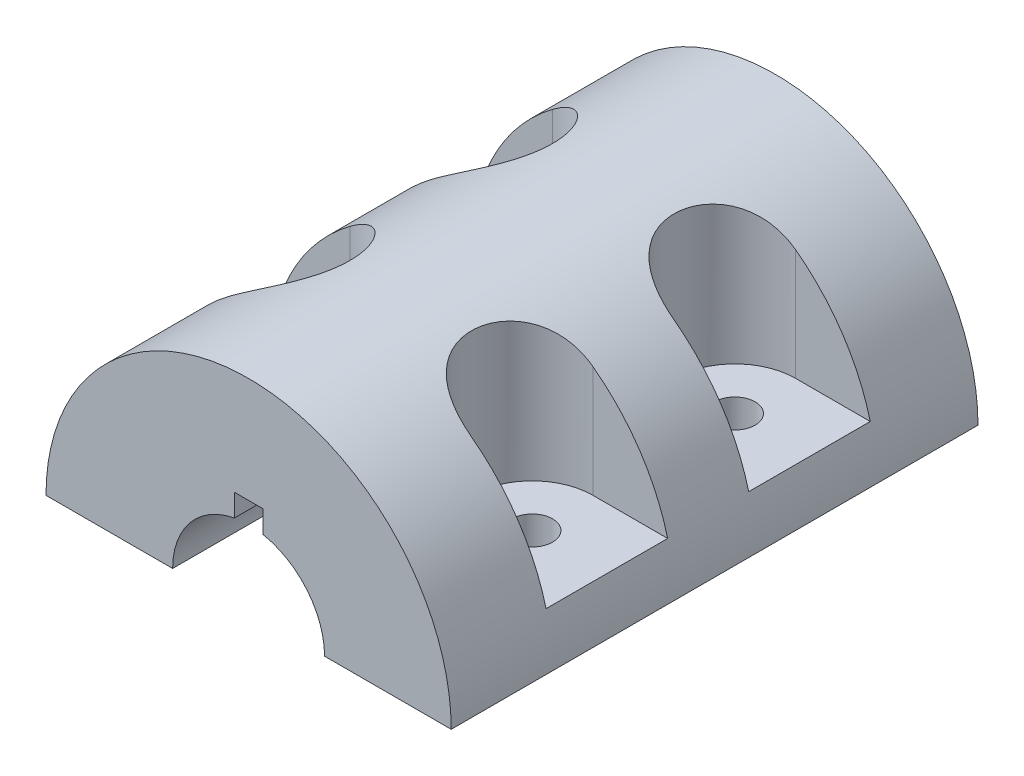
from build123d import *

# Parameters (mm, degrees)
HOUSING_BODY_DEPTH                     = 130
BOLT_START                             = 25
BOLT_POCKET_DEPTH                      = 260
BOLT_POCKET_MIRROR_RIGHT_COPY_1_DEPTH  = 260
BOLT_HOLE_SKETCH_R                     = 10
BOLT_HOLE_20_DEPTH                     = 260
BOLT_HOLE_MIRROR_RIGHT_COPY_1_SKETCH_R = 10
BOLT_HOLE_MIRROR_RIGHT_COPY_1_DEPTH    = 260
NOTCH_CUT_DEPTH                        = 296.972971894


with BuildPart() as part:
    # Housing Profile Sketch → Housing Body (new, symmetric)
    with BuildSketch(Plane.XY):
        with BuildLine():
            Line((-100, 0), (-37.5, 0))
            ThreePointArc((-37.5, 0), (0, 37.5), (37.5, 0))
            Line((37.5, 0), (100, 0))
            ThreePointArc((100, 0), (0, 100), (-100, 0))
        make_face()
    extrude(amount=HOUSING_BODY_DEPTH, both=True)

    # Bolt Pocket Sketch → Bolt Pocket (cut)
    with BuildSketch(Plane(origin=(0, 0, 0), x_dir=(1, 0, 0), z_dir=(0, 1, 0)).offset(BOLT_START)):
        with BuildLine():
            Line((-60, -20), (-100, -20))
            Line((-100, -20), (-100, -80))
            Line((-100, -80), (-60, -80))
            ThreePointArc((-60, -80), (-30, -50), (-60, -20))
        make_face()
    bolt_pocket = extrude(amount=BOLT_POCKET_DEPTH, mode=Mode.SUBTRACT)

    # Bolt Pocket Mirror Front: Bolt Pocket across plane
    add(bolt_pocket.mirror(Plane.XY), mode=Mode.SUBTRACT)

    # Bolt Pocket Mirror Right: Bolt Pocket across plane
    add(bolt_pocket.mirror(Plane(origin=(0, 0, 0), x_dir=(0, 0, 1), z_dir=(1, 0, 0))), mode=Mode.SUBTRACT)

    # Bolt Pocket Mirror Right copy 1 sketch → Bolt Pocket Mirror Right copy 1 (cut)
    with BuildSketch(Plane(origin=(0, 0, 0), x_dir=(-1, 0, 0), z_dir=(0, 1, 0)).offset(BOLT_START)):
        with BuildLine():
            Line((-60, -20), (-100, -20))
            Line((-100, -20), (-100, -80))
            Line((-100, -80), (-60, -80))
            ThreePointArc((-60, -80), (-30, -50), (-60, -20))
        make_face()
    extrude(amount=BOLT_POCKET_MIRROR_RIGHT_COPY_1_DEPTH, mode=Mode.SUBTRACT)

    # Bolt Hole Sketch → Bolt Hole Ø20 (cut)
    with BuildSketch(Plane(origin=(0, 25, 0), x_dir=(1, 0, 0), z_dir=(0, 1, 0))):
        with Locations(Location((-60, -50, 0), (0, 0, 270))):
            Circle(BOLT_HOLE_SKETCH_R)
    bolt_hole_20 = extrude(amount=-BOLT_HOLE_20_DEPTH, mode=Mode.SUBTRACT)

    # Bolt Hole Mirror Front: Bolt Hole Ø20 across plane
    add(bolt_hole_20.mirror(Plane.XY), mode=Mode.SUBTRACT)

    # Bolt Hole Mirror Right: Bolt Hole Ø20 across plane
    add(bolt_hole_20.mirror(Plane(origin=(0, 0, 0), x_dir=(0, 0, 1), z_dir=(1, 0, 0))), mode=Mode.SUBTRACT)

    # Bolt Hole Mirror Right copy 1 sketch → Bolt Hole Mirror Right copy 1 (cut)
    with BuildSketch(Plane(origin=(0, 25, 0), x_dir=(-1, 0, 0), z_dir=(0, 1, 0))):
        with Locations(Location((-60, -50, 0), (0, 0, 270))):
            Circle(BOLT_HOLE_MIRROR_RIGHT_COPY_1_SKETCH_R)
    extrude(amount=-BOLT_HOLE_MIRROR_RIGHT_COPY_1_DEPTH, mode=Mode.SUBTRACT)

    # Notch Sketch → Notch Cut (cut, through all)
    with BuildSketch(Plane(origin=(0, 0, -130), x_dir=(-1, 0, 0), z_dir=(0, 0, -1))):
        with BuildLine():
            Line((-7, 47.84087404), (7, 47.84087404))
            Line((7, 47.84087404), (7, 36.84087404))
            ThreePointArc((7, 36.84087404), (0, 37.5), (-7, 36.84087404))
            Line((-7, 36.84087404), (-7, 47.84087404))
        make_face()
    extrude(amount=-NOTCH_CUT_DEPTH, mode=Mode.SUBTRACT)


solid = part.part
